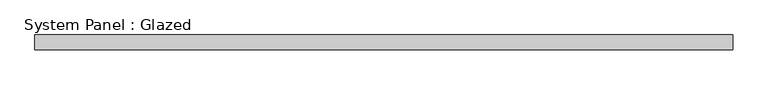
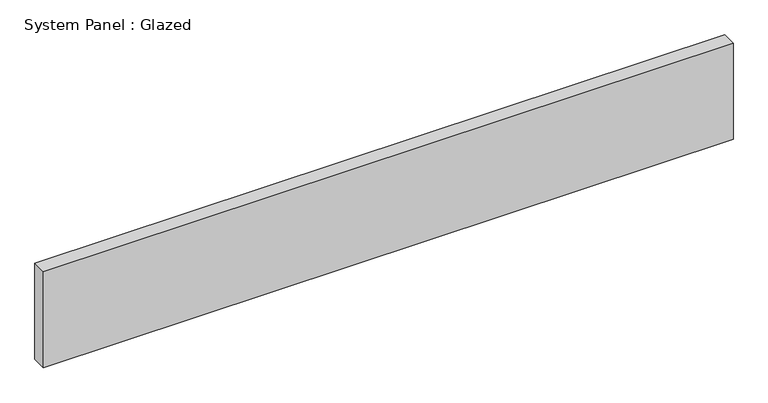
"""IFC4 building model written with IfcOpenShell, lengths in millimetres: plate geometry, System Panel : Glazed."""

from ifc_helpers import new_model, si_unit, origin, origin_with_axes, place, context, project, spatial, polyline, outline, extrude, source, transform, mapped, element, save


def system_panel_glazed_d1fc495d(model_context):
    return source(origin(), model_context, "Body", "SweptSolid", [
        extrude(outline(polyline([(603.2499999, 19.05), (-603.2499999, 19.05), (-603.2499999, 44.45), (603.2499999, 44.45), (603.2499999, 19.05)])), origin_with_axes(), (0.0, 0.0, 1.0), 177.8),
    ])


if __name__ == "__main__":
    model = new_model("IFC4")
    model_context = context("Model", 3, world=origin())
    ifc_project = project(units=[si_unit("LENGTHUNIT", "METRE", prefix="MILLI")], contexts=[model_context])
    site = spatial("IfcSite", under=ifc_project)
    building = spatial("IfcBuilding", under=site)
    placement = place(None, origin())
    system_panel_glazed_shape = system_panel_glazed_d1fc495d(model_context)
    element("IfcPlate", 1, ObjectType="System Panel : Glazed", at=placement, inside=building, context=model_context, shape_type="MappedRepresentation", body=[
        mapped(system_panel_glazed_shape, transform((0.0, 0.0, 0.0), x_axis=(1.0, 0.0, 0.0), y_axis=(0.0, 1.0, 0.0), z_axis=(0.0, 0.0, 1.0))),
    ])
    save(model, "model.ifc")

# Revit data of these elements
# Type "System Panel : Glazed"
#   Construction Type Id = "GSP4R"
#   Analytic Construction = "1/8 in Pilkington single glazing"
#   Visual Light Transmittance = 0.9
#   Solar Heat Gain Coefficient = 0.86
#   Heat Transfer Coefficient (U) = 1.18115 BTU/(h·ft²·°F)
#   Define Thermal Properties by = 1
# Element 1 (IfcPlate, "System Panel : Glazed")
#   Materials on its faces: "Glass"
# Materials
#   "Glass": class "Glass", colour RGB 0 128 192, transparency 0.75, Description = "Soda Lime Glass", Cost = 0
